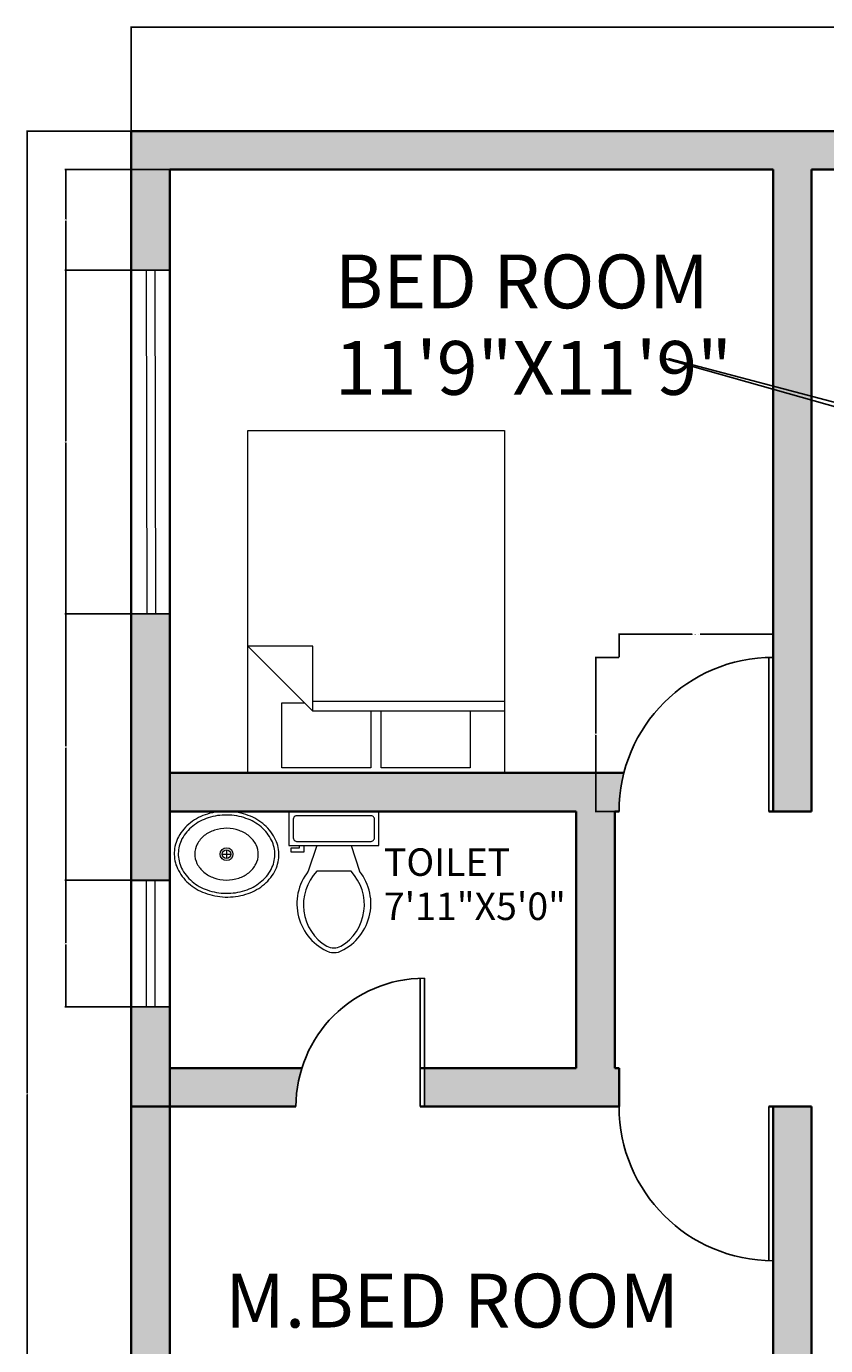
# Model space of a CAD drawing. Units: inches. Extents: x 582 to 1090, y 270 to 781.
# Tile 3 of 5: x 582 to 769, y 461 to 769. Entities that reach past the tile are written whole.
import ezdxf

# ---------------------------------------------------------------- set-up
doc = ezdxf.new("R2010")
doc.units = ezdxf.units.IN
doc.header["$MEASUREMENT"] = 0
for name, color, linetype, lineweight in [('A-ANNO-DIMS', 2, 'Continuous', 18), ('A-AREA-IDEN', 7, 'Continuous', 25), ('A-DOOR', 3, 'Continuous', 25), ('A-FLOR-FIXT', 9, 'Continuous', 18), ('A-FURN', 8, 'Continuous', 18), ('A-GLAZ', 4, 'Continuous', 18), ('A-WALL', 7, 'Continuous', 35)]:
    doc.layers.add(name, color=color, linetype=linetype, lineweight=lineweight)
doc.layers.add('A-WALL-PATT', color=9, linetype='Continuous', lineweight=13, true_color=0xc7c8ca)
doc.styles.get("Standard").update_dxf_attribs({"font": 'arial.ttf'})
doc.dimstyles.get("Standard").update_dxf_attribs({"dimtxt": 0.18, "dimasz": 0.18, "dimexe": 0.18, "dimexo": 0.0625, "dimgap": 0.09, "dimtad": 0, "dimtih": 1, "dimtoh": 1, "dimdec": 0, "dimzin": 0, "dimdsep": 46, "dimlunit": 3, "dimtxsty": 'Standard', "dimcen": 0.09, "dimadec": 0, "dimazin": 0, "dimtfac": 1, "dimtdec": 0, "dimtofl": 0, "dimtmove": 0, "dimatfit": 3, "dimfxl": 1, "dimtolj": 1, "dimtzin": 0, "dimarcsym": 0})

# ---------------------------------------------------------------- blocks, each defined once
blk = doc.blocks.new('Toilet - top')
for p, q in [((9.5, -6), (9.5, -2)), ((-10, -8.5), (-8, -8.5)), ((-10, -9.5), (-10, -8.5)), ((-8, -8.5), (-8, -8)), ((-7, -8), (-7, -9.5)), ((-4, -8), (-6, -14)), ((4, -8), (6, -14)), ((-7, -9.5), (-10, -9.5)), ((4, -14), (-4, -14))]:
    blk.add_line(p, q)
blk.add_lwpolyline([(10.5, -8), (10.5, 0), (-10.5, 0), (-10.5, -8)], close=True)
for points in [[(-9.5, -2), (-9.5, -6)], [(8.5, -1), (-8.5, -1)], [(-8.5, -7), (8.5, -7)]]:
    blk.add_lwpolyline(points)
for centre, radius, start, end in [((-8.62, -1.88), 0.884, 81.8699, 188.1301), ((8.62, -1.88), 0.884, 351.8699, 98.1301), ((-8.62, -6.12), 0.884, 171.8699, 278.1301), ((8.62, -6.12), 0.884, 261.8699, 8.1301), ((3.52, -21.58), 12.17, 141.4691, 247.9714), ((4.2, -21.82), 11.33, 136.3677, 238.9468), ((-3.52, -21.58), 12.17, 292.0284, 38.5307), ((-4.2, -21.82), 11.33, 301.053, 43.6321), ((0, -27.88), 4, 245.7318, 294.2682), ((0, -29), 4, 254.8605, 285.1395)]:
    blk.add_arc(centre, radius, start, end)
blk = doc.blocks.new('Sink - Oval top')
for p, q in [((-1, 0), (1, 0)), ((0, 1), (0, -1))]:
    blk.add_line(p, q)
for points in [[(-12.23, 0.39, 0.117634), (-11.46, -3.36, 0.104469), (-8.88, -6.8, 0.090016), (-5.08, -9.07, 0.08192), (-0.32, -10.02, 0.08192), (4.49, -9.38, 0.090016), (8.42, -7.36, 0.104469), (11.22, -4.09, 0.117634), (12.23, -0.39, 0.117634), (11.46, 3.36, 0.104469), (8.88, 6.8, 0.090016), (5.08, 9.07, 0.08192), (0.32, 10.02, 0.08192), (-4.49, 9.38, 0.090016), (-8.42, 7.36, 0.104469), (-11.22, 4.09, 0.117634)], [(-11.29, 0.16, 0.118622), (-10.52, -3.25, 0.104678), (-8.07, -6.36, 0.089562), (-4.54, -8.37, 0.081185), (-0.13, -9.15, 0.081185), (4.3, -8.49, 0.089562), (7.89, -6.58, 0.104678), (10.42, -3.55, 0.118622), (11.29, -0.16, 0.118622), (10.52, 3.25, 0.104678), (8.07, 6.36, 0.089562), (4.54, 8.37, 0.081185), (0.13, 9.15, 0.081185), (-4.3, 8.49, 0.089562), (-7.89, 6.58, 0.104678), (-10.42, 3.55, 0.118622)], [(-7.42, 0.08, 0.118283), (-6.91, -2.17, 0.104607), (-5.29, -4.21, 0.089718), (-2.97, -5.53, 0.081436), (-0.07, -6.04, 0.081436), (2.84, -5.59, 0.089718), (5.2, -4.33, 0.104607), (6.86, -2.32, 0.118283), (7.42, -0.08, 0.118283), (6.91, 2.17, 0.104607), (5.29, 4.21, 0.089718), (2.97, 5.53, 0.081436), (0.07, 6.04, 0.081436), (-2.84, 5.59, 0.089718), (-5.2, 4.33, 0.104607), (-6.86, 2.32, 0.118283)]]:
    blk.add_lwpolyline(points, format="xyb", close=True)
for radius in [1.5, 1]:
    blk.add_circle((0, 0), radius)
blk = doc.blocks.new('Bed - Queen')
for p, q in [((0, -80.00003), (0, 0)), ((0, 0), (59.99999, 0)), ((59.99999, 0), (59.99999, -80.00003)), ((7.99999, -1.2), (28.79998, -1.2)), ((7.99999, -14.4), (7.99999, -1.2)), ((28.79998, -1.2), (28.79998, -14.4)), ((31.19999, -1.2), (51.99999, -1.2)), ((31.19999, -14.4), (31.19999, -1.2)), ((51.99999, -1.2), (51.99999, -16.4)), ((0, -14.4), (44.8, -14.4)), ((59.99999, -29.6), (44.8, -14.4)), ((44.8, -14.4), (44.8, -29.6)), ((44.8, -16.8), (0, -16.8)), ((51.99999, -16.4), (46.79936, -16.4)), ((44.8, -29.6), (59.99999, -29.6)), ((59.99999, -80.00003), (0, -80.00003))]:
    blk.add_line(p, q)
blk = doc.blocks.new('DOOR-SINGLE-36IN')
for p, q in [((35, 0), (35, 36)), ((36, 0), (36, 36))]:
    blk.add_line(p, q)
blk.add_arc((36, 0), 36, 90, 180)
blk = doc.blocks.new('DOOR-SINGLE-30IN')
for p, q in [((29, 0), (29, 30)), ((30, 0), (30, 30))]:
    blk.add_line(p, q)
blk.add_arc((30, 0), 30, 90, 180)
blk = doc.blocks.new('*D26')
at = {"layer": 'A-ANNO-DIMS', "color": 0, "lineweight": -2, "transparency": 16777216}
for p, q in [((720.8, 621.51), (720.8, 627.03)), ((720.98, 626.85), (737.87, 626.85)), ((756.62, 626.85), (739.74, 626.85)), ((756.8, 621.51), (756.8, 627.03))]:
    blk.add_line(p, q, dxfattribs=at)
at = {"layer": 'A-ANNO-DIMS', "color": 0, "transparency": 16777216}
for points in [[(720.98, 626.88), (720.98, 626.82), (720.8, 626.85)], [(756.62, 626.88), (756.62, 626.82), (756.8, 626.85)]]:
    blk.add_solid(points, dxfattribs=at)
at = {"layer": 'Defpoints', "color": 0, "transparency": 16777216}
for p in [(756.8, 626.85), (720.8, 621.45), (756.8, 621.45)]:
    blk.add_point(p, dxfattribs=at)
at = {"layer": 'A-ANNO-DIMS', "color": 0, "transparency": 16777216, "insert": (738.8, 626.85), "char_height": 0.18, "attachment_point": 5}
blk.add_mtext('\\A1;DOOR 36 TYP.', dxfattribs=at)
blk = doc.blocks.new('*D27')
at = {"layer": 'A-ANNO-DIMS', "color": 0, "lineweight": -2, "transparency": 16777216}
for p, q in [((720.74, 621.45), (715.22, 621.45)), ((715.4, 621.27), (715.4, 603.63)), ((715.4, 585.63), (715.4, 603.26)), ((720.74, 585.45), (715.22, 585.45))]:
    blk.add_line(p, q, dxfattribs=at)
at = {"layer": 'A-ANNO-DIMS', "color": 0, "transparency": 16777216}
for points in [[(715.37, 621.27), (715.43, 621.27), (715.4, 621.45)], [(715.37, 585.63), (715.43, 585.63), (715.4, 585.45)]]:
    blk.add_solid(points, dxfattribs=at)
at = {"layer": 'Defpoints', "color": 0, "transparency": 16777216}
for p in [(715.4, 621.45), (720.8, 621.45), (720.8, 585.45)]:
    blk.add_point(p, dxfattribs=at)
at = {"layer": 'A-ANNO-DIMS', "color": 0, "transparency": 16777216, "insert": (715.4, 603.45), "char_height": 0.18, "attachment_point": 5}
blk.add_mtext('\\A1;36 TYP.', dxfattribs=at)
blk = doc.blocks.new('*D34')
at = {"layer": 'A-ANNO-DIMS', "color": 0, "lineweight": -2, "transparency": 16777216}
for p, q in [((606.8, 744.51), (606.8, 768.93)), ((606.98, 768.75), (836.01, 768.75)), ((1065.62, 768.75), (836.6, 768.75)), ((1065.8, 744.51), (1065.8, 768.93))]:
    blk.add_line(p, q, dxfattribs=at)
at = {"layer": 'A-ANNO-DIMS', "color": 0, "transparency": 16777216}
for points in [[(606.98, 768.78), (606.98, 768.72), (606.8, 768.75)], [(1065.62, 768.78), (1065.62, 768.72), (1065.8, 768.75)]]:
    blk.add_solid(points, dxfattribs=at)
at = {"layer": 'Defpoints', "color": 0, "transparency": 16777216}
for p in [(1065.8, 768.75), (606.8, 744.45), (1065.8, 744.45)]:
    blk.add_point(p, dxfattribs=at)
at = {"layer": 'A-ANNO-DIMS', "color": 0, "transparency": 16777216, "insert": (836.3, 768.75), "char_height": 0.18, "attachment_point": 5}
blk.add_mtext('\\A1;459', dxfattribs=at)
blk = doc.blocks.new('*D36')
at = {"layer": 'A-ANNO-DIMS', "color": 0, "lineweight": -2, "transparency": 16777216}
for p, q in [((606.74, 744.45), (582.32, 744.45)), ((582.5, 744.27), (582.5, 519.62)), ((582.5, 294.62), (582.5, 519.26)), ((756.74, 294.44), (582.32, 294.44))]:
    blk.add_line(p, q, dxfattribs=at)
at = {"layer": 'A-ANNO-DIMS', "color": 0, "transparency": 16777216}
for points in [[(582.47, 744.27), (582.53, 744.27), (582.5, 744.45)], [(582.47, 294.62), (582.53, 294.62), (582.5, 294.44)]]:
    blk.add_solid(points, dxfattribs=at)
at = {"layer": 'Defpoints', "color": 0, "transparency": 16777216}
for p in [(582.5, 744.45), (606.8, 744.45), (756.8, 294.44)]:
    blk.add_point(p, dxfattribs=at)
at = {"layer": 'A-ANNO-DIMS', "color": 0, "transparency": 16777216, "insert": (582.5, 519.44), "char_height": 0.18, "attachment_point": 5}
blk.add_mtext('\\A1;450', dxfattribs=at)
blk = doc.blocks.new('*D48')
at = {"layer": 'A-ANNO-DIMS', "color": 0, "lineweight": -2, "transparency": 16777216}
for p, q in [((615.74, 735.45), (591.32, 735.45)), ((591.5, 735.27), (591.5, 723.87)), ((591.5, 712.12), (591.5, 723.51)), ((615.74, 711.94), (591.32, 711.94))]:
    blk.add_line(p, q, dxfattribs=at)
at = {"layer": 'A-ANNO-DIMS', "color": 0, "transparency": 16777216}
for points in [[(591.47, 735.27), (591.53, 735.27), (591.5, 735.45)], [(591.47, 712.12), (591.53, 712.12), (591.5, 711.94)]]:
    blk.add_solid(points, dxfattribs=at)
at = {"layer": 'Defpoints', "color": 0, "transparency": 16777216}
for p in [(591.5, 735.45), (615.8, 735.45), (615.8, 711.94)]:
    blk.add_point(p, dxfattribs=at)
at = {"layer": 'A-ANNO-DIMS', "color": 0, "transparency": 16777216, "insert": (591.5, 723.69), "char_height": 0.18, "attachment_point": 5}
blk.add_mtext('\\A1;23.51', dxfattribs=at)
blk = doc.blocks.new('*D49')
at = {"layer": 'A-ANNO-DIMS', "color": 0, "lineweight": -2, "transparency": 16777216}
for p, q in [((615.74, 711.94), (591.32, 711.94)), ((591.5, 711.76), (591.5, 671.98)), ((591.5, 631.83), (591.5, 671.61)), ((615.74, 631.65), (591.32, 631.65))]:
    blk.add_line(p, q, dxfattribs=at)
at = {"layer": 'A-ANNO-DIMS', "color": 0, "transparency": 16777216}
for points in [[(591.47, 711.76), (591.53, 711.76), (591.5, 711.94)], [(591.47, 631.83), (591.53, 631.83), (591.5, 631.65)]]:
    blk.add_solid(points, dxfattribs=at)
at = {"layer": 'Defpoints', "color": 0, "transparency": 16777216}
for p in [(591.5, 711.94), (615.8, 711.94), (615.8, 631.65)]:
    blk.add_point(p, dxfattribs=at)
at = {"layer": 'A-ANNO-DIMS', "color": 0, "transparency": 16777216, "insert": (591.5, 671.79), "char_height": 0.18, "attachment_point": 5}
blk.add_mtext('\\A1;80.29', dxfattribs=at)
blk = doc.blocks.new('*D50')
at = {"layer": 'A-ANNO-DIMS', "color": 0, "lineweight": -2, "transparency": 16777216}
for p, q in [((615.74, 631.65), (591.32, 631.65)), ((591.5, 631.47), (591.5, 600.68)), ((591.5, 569.52), (591.5, 600.31)), ((615.74, 569.34), (591.32, 569.34))]:
    blk.add_line(p, q, dxfattribs=at)
at = {"layer": 'A-ANNO-DIMS', "color": 0, "transparency": 16777216}
for points in [[(591.47, 631.47), (591.53, 631.47), (591.5, 631.65)], [(591.47, 569.52), (591.53, 569.52), (591.5, 569.34)]]:
    blk.add_solid(points, dxfattribs=at)
at = {"layer": 'Defpoints', "color": 0, "transparency": 16777216}
for p in [(591.5, 631.65), (615.8, 631.65), (615.8, 569.34)]:
    blk.add_point(p, dxfattribs=at)
at = {"layer": 'A-ANNO-DIMS', "color": 0, "transparency": 16777216, "insert": (591.5, 600.49), "char_height": 0.18, "attachment_point": 5}
blk.add_mtext('\\A1;62.31', dxfattribs=at)
blk = doc.blocks.new('*D51')
at = {"layer": 'A-ANNO-DIMS', "color": 0, "lineweight": -2, "transparency": 16777216}
for p, q in [((615.74, 569.34), (591.32, 569.34)), ((591.5, 569.16), (591.5, 554.73)), ((591.5, 539.95), (591.5, 554.37)), ((615.74, 539.77), (591.32, 539.77))]:
    blk.add_line(p, q, dxfattribs=at)
at = {"layer": 'A-ANNO-DIMS', "color": 0, "transparency": 16777216}
for points in [[(591.47, 569.16), (591.53, 569.16), (591.5, 569.34)], [(591.47, 539.95), (591.53, 539.95), (591.5, 539.77)]]:
    blk.add_solid(points, dxfattribs=at)
at = {"layer": 'Defpoints', "color": 0, "transparency": 16777216}
for p in [(591.5, 569.34), (615.8, 569.34), (615.8, 539.77)]:
    blk.add_point(p, dxfattribs=at)
at = {"layer": 'A-ANNO-DIMS', "color": 0, "transparency": 16777216, "insert": (591.5, 554.55), "char_height": 0.18, "attachment_point": 5}
blk.add_mtext('\\A1;29.57', dxfattribs=at)
blk = doc.blocks.new('*D75')
at = {"layer": 'A-ANNO-DIMS', "color": 0, "lineweight": -2, "transparency": 16777216}
for p, q in [((732.37, 691.29), (782.48, 678.04)), ((866.37, 655.84), (866.55, 655.84)), ((866.46, 655.75), (866.46, 655.93))]:
    blk.add_line(p, q, dxfattribs=at)
at = {"layer": 'A-ANNO-DIMS', "color": 0, "transparency": 16777216}
blk.add_solid([(782.49, 678.07), (782.47, 678.01), (782.66, 678)], dxfattribs=at)
at = {"layer": 'Defpoints', "color": 0, "transparency": 16777216}
for p in [(782.66, 678), (866.46, 655.84)]:
    blk.add_point(p, dxfattribs=at)
at = {"layer": 'A-ANNO-DIMS', "color": 0, "transparency": 16777216, "insert": (731.89, 691.29), "char_height": 0.18, "attachment_point": 5}
blk.add_mtext('\\A1;R86.69', dxfattribs=at)
blk = doc.blocks.new('*D76')
at = {"layer": 'A-ANNO-DIMS', "color": 0, "lineweight": -2, "transparency": 16777216}
for p, q in [((731.17, 691.3), (731.35, 691.3)), ((731.35, 691.3), (778.37, 678.05)), ((857.11, 655.84), (857.29, 655.84)), ((857.2, 655.75), (857.2, 655.93))]:
    blk.add_line(p, q, dxfattribs=at)
at = {"layer": 'A-ANNO-DIMS', "color": 0, "transparency": 16777216}
blk.add_solid([(778.38, 678.08), (778.37, 678.02), (778.55, 678)], dxfattribs=at)
at = {"layer": 'Defpoints', "color": 0, "transparency": 16777216}
for p in [(778.55, 678), (857.2, 655.84)]:
    blk.add_point(p, dxfattribs=at)
at = {"layer": 'A-ANNO-DIMS', "color": 0, "transparency": 16777216, "insert": (730.7, 691.3), "char_height": 0.18, "attachment_point": 5}
blk.add_mtext('\\A1;R81.72', dxfattribs=at)

msp = doc.modelspace()

# ---------------------------------------------------------------- hatches: boundary and pattern name
at = {"layer": 'A-WALL-PATT'}
h = msp.add_hatch(color=256, dxfattribs=at)
h.dxf.hatch_style = 1
h.paths.add_polyline_path([(867.8047, 744.446), (765.8047, 744.446), (606.8047, 744.446), (606.8047, 711.9379), (615.8047, 711.9379), (615.8047, 735.446), (756.8047, 735.446), (756.8047, 585.446), (765.8047, 585.446), (765.8047, 735.446), (868.9478, 735.446, -0.06325422)])
h.paths.add_polyline_path([(1065.8047, 744.446), (912.8047, 744.446), (903.8047, 744.446), (903.8047, 708.446), (903.8047, 594.446), (903.8047, 564.6071), (912.8047, 564.6071), (912.8047, 600.6071), (912.8047, 735.446), (1056.8047, 735.446), (1056.8047, 720.2375), (1065.8047, 720.2375)])
h.paths.add_polyline_path([(1065.8047, 632.4383), (1056.8047, 632.4383), (1056.8047, 594.446), (1056.8047, 584.9343), (1065.8047, 584.9343), (1065.8047, 594.446)], flags=17)
h.paths.add_polyline_path([(1056.8047, 603.446), (951.8047, 603.446), (951.8047, 594.446), (1056.8047, 594.446)], flags=17)
h.paths.add_polyline_path([(1065.8047, 525.446), (1065.8047, 550.2593), (1056.8047, 550.2593), (1056.8047, 534.446), (960.8047, 534.446), (960.8047, 565.946, -0.07397332), (952.1262, 564.6071), (951.8047, 564.6071), (951.8047, 495.446, -0.07632083), (960.8047, 494.0641), (960.8047, 525.446), (1056.8047, 525.446), (1056.8047, 508.8565), (1065.8047, 508.8565)])
h.paths.add_polyline_path([(1065.8047, 478.2143), (1056.8047, 478.2143), (1056.8047, 465.446), (951.8047, 465.446), (951.8047, 456.446), (1056.8047, 456.446), (1056.8047, 420.446), (1065.8047, 420.446), (1065.8047, 456.446)])
h.paths.add_polyline_path([(1065.8047, 420.446), (1056.8047, 420.446), (1017.8047, 420.446), (1017.8047, 456.446), (1008.8047, 456.446), (1008.8047, 411.446), (1038.8047, 411.446), (1065.8047, 411.446)])
h.paths.add_polyline_path([(1065.8047, 411.446), (1056.8047, 411.446), (1056.8047, 327.446), (1065.8047, 327.446)])
h.paths.add_polyline_path([(1065.8047, 327.446), (1056.8047, 327.446), (1017.8047, 327.446), (1017.8047, 382.8278, -0.07632083), (1008.8047, 381.446), (1008.8047, 327.446), (983.7348, 327.446), (983.7348, 318.446), (1065.8047, 318.446)])
h.paths.add_polyline_path([(946.9624, 327.446), (918.8047, 327.446), (918.8047, 369.8742), (918.8047, 459.446), (909.8047, 459.446), (909.8047, 369.8742), (909.8047, 318.446), (946.9624, 318.446)])
h.paths.add_polyline_path([(918.8047, 318.446), (909.8047, 318.446), (909.8047, 303.4372), (765.8047, 303.4372), (765.8047, 327.446), (756.8047, 327.446), (756.8047, 294.4372), (918.8047, 294.4372)])
h.paths.add_polyline_path([(909.8047, 378.8742), (882.3477, 378.8742), (882.3477, 347.0959), (889.3299, 347.0959), (889.3299, 369.8742), (909.8047, 369.8742)])
h.paths.add_polyline_path([(779.4225, 378.8742), (765.8047, 378.8742), (765.8047, 369.8742), (779.4225, 369.8742)])
h.paths.add_polyline_path([(765.8047, 516.446), (756.8047, 516.446), (756.8047, 480.446), (756.8047, 336.446), (724.1731, 336.446), (724.1731, 327.446), (765.8047, 327.446), (765.8047, 369.8742), (765.8047, 378.8742)])
h.paths.add_polyline_path([(615.8047, 516.446), (606.8047, 516.446), (606.8047, 327.446), (637.062, 327.446), (637.062, 336.446), (615.8047, 336.446)])
h.paths.add_polyline_path([(615.8047, 631.6498), (606.8047, 631.6498), (606.8047, 585.446), (606.8047, 569.338), (615.8047, 569.338), (615.8047, 585.446), (615.8047, 594.446)])
h.paths.add_polyline_path([(721.9478, 594.446), (615.8047, 594.446), (615.8047, 585.446), (627.9505, 585.446, -0.03261849), (629.8936, 585.446), (710.8047, 585.446), (710.8047, 525.446), (675.3033, 525.446), (675.3033, 516.446), (719.8047, 516.446), (720.8047, 516.446), (720.8047, 525.446), (719.8047, 525.446), (719.8047, 585.446), (720.8047, 585.446, -0.06325422)])
h.paths.add_polyline_path([(646.6852, 525.446), (615.8047, 525.446), (615.8047, 516.446), (645.3033, 516.446, -0.07632083)])
h.paths.add_polyline_path([(615.8047, 525.446), (615.8047, 539.7667), (606.8047, 539.7667), (606.8047, 516.446), (615.8047, 516.446)])

# ---------------------------------------------------------------- linework, layer by layer
at = {"layer": 'A-DOOR'}
for p, q in [((675.3033, 516.446), (674.3033, 516.446)), ((756.8047, 516.446), (755.8047, 516.446))]:
    msp.add_line(p, q, dxfattribs=at)
at = {"layer": 'A-GLAZ'}
for p, q in [((606.8047, 711.9379), (615.8047, 711.9379)), ((610.3047, 711.9361), (610.4512, 631.6479)), ((612.3047, 711.9397), (612.4512, 631.6516)), ((615.8047, 631.6498), (606.8047, 631.6498)), ((611.4512, 631.6498), (615.8047, 631.6498)), ((606.8047, 569.338), (615.8047, 569.338)), ((610.3047, 569.338), (610.3047, 539.7667)), ((612.3047, 569.338), (612.3047, 539.7667)), ((615.8047, 539.7667), (606.8047, 539.7667)), ((611.3047, 539.7667), (615.8047, 539.7667))]:
    msp.add_line(p, q, dxfattribs=at)
at = {"layer": 'A-WALL'}
for p, q in [((606.8047, 744.446), (765.8047, 744.446)), ((606.8047, 744.446), (606.8047, 585.446)), ((912.8047, 744.446), (765.8047, 744.446)), ((615.8047, 735.446), (615.8047, 594.446)), ((615.8047, 735.446), (756.8047, 735.446)), ((756.8047, 735.446), (756.8047, 585.446)), ((765.8047, 735.446), (765.8047, 585.446)), ((765.8047, 735.446), (868.9478, 735.446)), ((721.9478, 594.446), (615.8047, 594.446)), ((615.8047, 594.446), (615.8047, 585.446)), ((606.8047, 585.446), (606.8047, 516.446)), ((615.8047, 585.446), (615.8047, 525.446)), ((710.8047, 585.446), (615.8047, 585.446)), ((710.8047, 525.446), (710.8047, 585.446)), ((719.8047, 525.446), (719.8047, 585.446)), ((720.8047, 585.446), (719.8047, 585.446)), ((765.8047, 585.446), (755.8047, 585.446)), ((615.8047, 525.446), (646.6852, 525.446)), ((615.8047, 525.446), (615.8047, 516.446)), ((674.3033, 525.446), (710.8047, 525.446)), ((720.8047, 525.446), (719.8047, 525.446)), ((720.8047, 516.446), (720.8047, 525.446)), ((606.8047, 516.446), (645.3033, 516.446)), ((606.8047, 516.446), (606.8047, 327.446)), ((615.8047, 516.446), (615.8047, 336.446)), ((674.3033, 516.446), (719.8047, 516.446)), ((720.8047, 516.446), (719.8047, 516.446)), ((765.8047, 516.446), (755.8047, 516.446)), ((756.8047, 336.446), (756.8047, 516.446)), ((765.8047, 327.446), (765.8047, 516.446)), ((765.8047, 516.446), (765.8047, 396.446))]:
    msp.add_line(p, q, dxfattribs=at)

# ---------------------------------------------------------------- block references
at = {"layer": 'A-DOOR'}
for name, p in [('DOOR-SINGLE-36IN', (720.805, 585.446)), ('DOOR-SINGLE-30IN', (645.303, 516.446))]:
    msp.add_blockref(name, p, dxfattribs=at)
at = {"layer": 'A-DOOR', "extrusion": (0, 0, -1), "zscale": -1, "rotation": 180}
msp.add_blockref('DOOR-SINGLE-36IN', (-720.805, 516.4459), dxfattribs=at)
at = {"layer": 'A-FLOR-FIXT'}
for name, p in [('Sink - Oval top', (629.0795, 575.4541)), ('Toilet - top', (654.1624, 585.446))]:
    msp.add_blockref(name, p, dxfattribs=at)
at = {"layer": 'A-FURN', "rotation": 180}
msp.add_blockref('Bed - Queen', (694.021, 594.446), dxfattribs=at)

# ---------------------------------------------------------------- texts
at = {"layer": 'A-ANNO-DIMS'}
for s, height, p in [('11\'9"X11\'9"', 12.580749, (654.3857, 682.8136)), ('7\'11"X5\'0"', 6.42605, (665.846, 560.0596))]:
    msp.add_text(s, height=height, dxfattribs=at).set_placement(p)
at = {"layer": 'A-AREA-IDEN'}
for s, height, p in [('BED ROOM', 12.58075, (654.3857, 703.0234)), ('TOILET', 6.42605, (665.846, 570.3825)), ('M.BED ROOM', 12.58075, (628.7733, 464.8126))]:
    msp.add_text(s, height=height, dxfattribs=at).set_placement(p)

# ---------------------------------------------------------------- dimensions: what is measured, and where the dimension line sits
at = {"layer": 'A-ANNO-DIMS'}
dim = msp.add_linear_dim(base=(1065.8047, 768.746), p1=(606.8047, 744.446), p2=(1065.8047, 744.446), dimstyle='Standard', override={"dimdec": 0, "dimlfac": 1, "dimrnd": 0, "dimzin": 0, "dimdsep": 46, "dimlunit": 2}, dxfattribs=at)
dim.commit()
dim.dimension.update_dxf_attribs({"geometry": '*D34', "text_midpoint": (836.3047, 768.746)})
for base, p1, p2, override, picture, middle in [((582.5047, 744.446), (756.8047, 294.4372), (606.8047, 744.446), {"dimdec": 0, "dimlfac": 1, "dimrnd": 0, "dimzin": 0, "dimdsep": 46, "dimlunit": 2}, '*D36', (582.5047, 519.4416)), ((591.5047, 735.446), (615.8047, 711.9379), (615.8047, 735.446), {"dimdec": 2, "dimlfac": 1, "dimrnd": 0, "dimzin": 0, "dimdsep": 46, "dimlunit": 2}, '*D48', (591.5047, 723.6919)), ((591.5047, 711.9379), (615.8047, 631.6498), (615.8047, 711.9379), {"dimdec": 2, "dimlfac": 1, "dimrnd": 0, "dimzin": 0, "dimdsep": 46, "dimlunit": 2}, '*D49', (591.5047, 671.7938)), ((591.5047, 631.6498), (615.8047, 569.338), (615.8047, 631.6498), {"dimdec": 2, "dimlfac": 1, "dimrnd": 0, "dimzin": 0, "dimdsep": 46, "dimlunit": 2}, '*D50', (591.5047, 600.4939)), ((591.5047, 569.338), (615.8047, 539.7667), (615.8047, 569.338), {"dimdec": 2, "dimlfac": 1, "dimrnd": 0, "dimzin": 0, "dimdsep": 46, "dimlunit": 2}, '*D51', (591.5047, 554.5524))]:
    dim = msp.add_linear_dim(base=base, p1=p1, p2=p2, angle=90, dimstyle='Standard', override=override, dxfattribs=at)
    dim.commit()
    dim.dimension.update_dxf_attribs({"geometry": picture, "text_midpoint": middle})
for center, mpoint, picture, middle in [((857.2034, 655.8447), (778.5479, 678.0034), '*D76', (730.6957, 691.2986)), ((866.4635, 655.8447), (782.6557, 677.9959), '*D75', (732.371, 691.2866))]:
    dim = msp.add_radius_dim(center=center, mpoint=mpoint, dimstyle='Standard', override={"dimdec": 2, "dimlfac": 1, "dimrnd": 0, "dimzin": 0, "dimdsep": 46, "dimlunit": 2}, dxfattribs=at)
    dim.commit()
    dim.dimension.update_dxf_attribs({"geometry": picture, "text_midpoint": middle, "dimtype": 164})
dim = msp.add_linear_dim(base=(756.8047, 626.846), p1=(720.8047, 621.446), p2=(756.8047, 621.446), text='DOOR <> TYP.', dimstyle='Standard', override={"dimdec": 0, "dimlfac": 1, "dimrnd": 0, "dimzin": 0, "dimdsep": 46, "dimlunit": 2}, dxfattribs=at)
dim.commit()
dim.dimension.update_dxf_attribs({"geometry": '*D26', "text_midpoint": (738.8047, 626.846)})
dim = msp.add_linear_dim(base=(715.4047, 621.446), p1=(720.8047, 585.446), p2=(720.8047, 621.446), angle=90, text='<> TYP.', dimstyle='Standard', override={"dimdec": 0, "dimlfac": 1, "dimrnd": 0, "dimzin": 0, "dimdsep": 46, "dimlunit": 2}, dxfattribs=at)
dim.commit()
dim.dimension.update_dxf_attribs({"geometry": '*D27', "text_midpoint": (715.4047, 603.446)})

doc.saveas('drawing.dxf')
